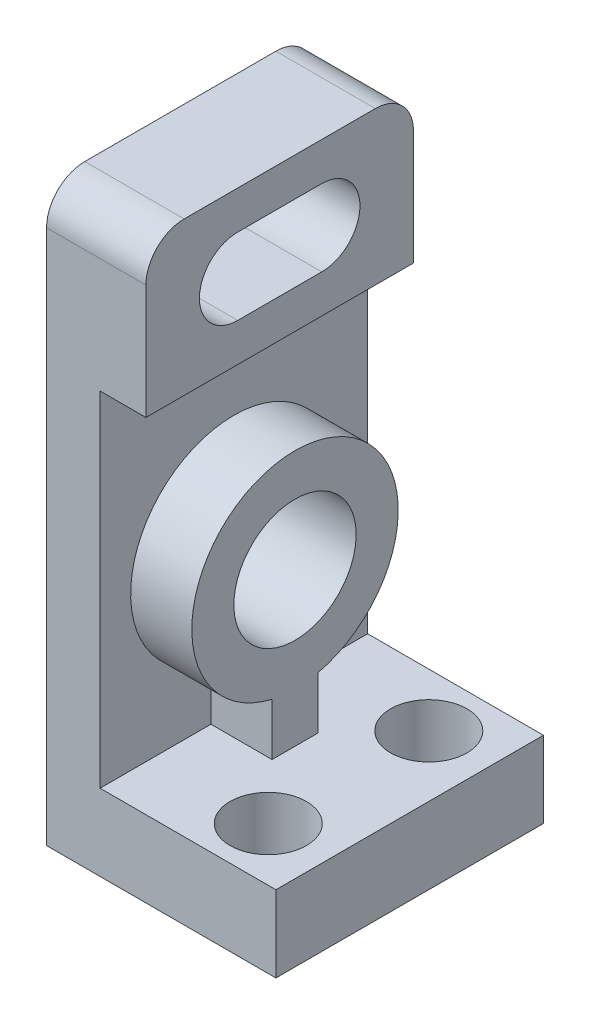
ISO-10303-21;
HEADER;
FILE_DESCRIPTION(('STEP AP214'),'2;1');
FILE_NAME('part.step','',(''),(''),'','','');
FILE_SCHEMA(('AUTOMOTIVE_DESIGN { 1 0 10303 214 1 1 1 1 }'));
ENDSEC;
DATA;
#1=APPLICATION_CONTEXT('core data for automotive mechanical design processes');
#2=APPLICATION_PROTOCOL_DEFINITION('international standard','automotive_design',2000,#1);
#3=PRODUCT_CONTEXT('',#1,'mechanical');
#4=PRODUCT('Part','Part','',(#3));
#5=PRODUCT_RELATED_PRODUCT_CATEGORY('part','',(#4));
#6=PRODUCT_DEFINITION_FORMATION('','',#4);
#7=PRODUCT_DEFINITION_CONTEXT('part definition',#1,'design');
#8=PRODUCT_DEFINITION('design','',#6,#7);
#9=PRODUCT_DEFINITION_SHAPE('','',#8);
#10=(LENGTH_UNIT() NAMED_UNIT(*) SI_UNIT(.MILLI.,.METRE.));
#11=(NAMED_UNIT(*) PLANE_ANGLE_UNIT() SI_UNIT($,.RADIAN.));
#12=(NAMED_UNIT(*) SI_UNIT($,.STERADIAN.) SOLID_ANGLE_UNIT());
#13=UNCERTAINTY_MEASURE_WITH_UNIT(LENGTH_MEASURE(1.E-05),#10,'distance_accuracy_value','');
#14=(GEOMETRIC_REPRESENTATION_CONTEXT(3) GLOBAL_UNCERTAINTY_ASSIGNED_CONTEXT((#13)) GLOBAL_UNIT_ASSIGNED_CONTEXT((#10,
#11,#12)) REPRESENTATION_CONTEXT('',''));
#15=CARTESIAN_POINT('',(0.,0.,0.));
#16=DIRECTION('',(0.,0.,1.));
#17=DIRECTION('',(1.,0.,0.));
#18=AXIS2_PLACEMENT_3D('',#15,#16,#17);
#19=CARTESIAN_POINT('',(7.,10.,17.5));
#20=DIRECTION('',(0.,-1.,0.));
#21=DIRECTION('',(0.,0.,-1.));
#22=AXIS2_PLACEMENT_3D('',#19,#20,#21);
#23=PLANE('',#22);
#24=CARTESIAN_POINT('',(22.,10.,-10.5));
#25=DIRECTION('',(0.,1.,0.));
#26=DIRECTION('',(0.,0.,1.));
#27=AXIS2_PLACEMENT_3D('',#24,#25,#26);
#28=CIRCLE('',#27,5.);
#29=CARTESIAN_POINT('',(22.,10.,-5.5));
#30=VERTEX_POINT('',#29);
#31=EDGE_CURVE('E244',#30,#30,#28,.T.);
#32=ORIENTED_EDGE('',*,*,#31,.F.);
#33=EDGE_LOOP('',(#32));
#34=FACE_BOUND('',#33,.T.);
#35=CARTESIAN_POINT('',(22.,10.,10.5));
#36=DIRECTION('',(0.,1.,0.));
#37=DIRECTION('',(0.,0.,1.));
#38=AXIS2_PLACEMENT_3D('',#35,#36,#37);
#39=CIRCLE('',#38,5.);
#40=CARTESIAN_POINT('',(22.,10.,15.5));
#41=VERTEX_POINT('',#40);
#42=EDGE_CURVE('E236',#41,#41,#39,.T.);
#43=ORIENTED_EDGE('',*,*,#42,.F.);
#44=EDGE_LOOP('',(#43));
#45=FACE_BOUND('',#44,.T.);
#46=DIRECTION('',(-1.,0.,0.));
#47=VECTOR('',#46,1.);
#48=CARTESIAN_POINT('',(15.,10.,-3.));
#49=LINE('',#48,#47);
#50=CARTESIAN_POINT('',(15.,10.,-3.));
#51=VERTEX_POINT('',#50);
#52=CARTESIAN_POINT('',(7.,10.,-3.));
#53=VERTEX_POINT('',#52);
#54=EDGE_CURVE('E226',#51,#53,#49,.T.);
#55=ORIENTED_EDGE('',*,*,#54,.F.);
#56=DIRECTION('',(0.,0.,-1.));
#57=VECTOR('',#56,1.);
#58=CARTESIAN_POINT('',(15.,10.,3.));
#59=LINE('',#58,#57);
#60=CARTESIAN_POINT('',(15.,10.,3.));
#61=VERTEX_POINT('',#60);
#62=EDGE_CURVE('E212',#61,#51,#59,.T.);
#63=ORIENTED_EDGE('',*,*,#62,.F.);
#64=DIRECTION('',(-1.,0.,0.));
#65=VECTOR('',#64,1.);
#66=CARTESIAN_POINT('',(15.,10.,3.));
#67=LINE('',#66,#65);
#68=CARTESIAN_POINT('',(7.,10.,3.));
#69=VERTEX_POINT('',#68);
#70=EDGE_CURVE('E231',#61,#69,#67,.T.);
#71=ORIENTED_EDGE('',*,*,#70,.T.);
#72=DIRECTION('',(0.,0.,-1.));
#73=VECTOR('',#72,1.);
#74=CARTESIAN_POINT('',(7.,10.,17.5));
#75=LINE('',#74,#73);
#76=CARTESIAN_POINT('',(7.,10.,17.5));
#77=VERTEX_POINT('',#76);
#78=EDGE_CURVE('E300',#77,#69,#75,.T.);
#79=ORIENTED_EDGE('',*,*,#78,.F.);
#80=DIRECTION('',(-1.,0.,0.));
#81=VECTOR('',#80,1.);
#82=CARTESIAN_POINT('',(7.,10.,17.5));
#83=LINE('',#82,#81);
#84=CARTESIAN_POINT('',(30.,10.,17.5));
#85=VERTEX_POINT('',#84);
#86=EDGE_CURVE('E258',#85,#77,#83,.T.);
#87=ORIENTED_EDGE('',*,*,#86,.F.);
#88=DIRECTION('',(0.,0.,-1.));
#89=VECTOR('',#88,1.);
#90=CARTESIAN_POINT('',(30.,10.,17.5));
#91=LINE('',#90,#89);
#92=CARTESIAN_POINT('',(30.,10.,-17.5));
#93=VERTEX_POINT('',#92);
#94=EDGE_CURVE('E304',#85,#93,#91,.T.);
#95=ORIENTED_EDGE('',*,*,#94,.T.);
#96=DIRECTION('',(-1.,0.,0.));
#97=VECTOR('',#96,1.);
#98=CARTESIAN_POINT('',(7.,10.,-17.5));
#99=LINE('',#98,#97);
#100=CARTESIAN_POINT('',(7.,10.,-17.5));
#101=VERTEX_POINT('',#100);
#102=EDGE_CURVE('E275',#93,#101,#99,.T.);
#103=ORIENTED_EDGE('',*,*,#102,.T.);
#104=EDGE_CURVE('E299',#53,#101,#75,.T.);
#105=ORIENTED_EDGE('',*,*,#104,.F.);
#106=EDGE_LOOP('',(#55,#63,#71,#79,#87,#95,#103,#105));
#107=FACE_BOUND('',#106,.T.);
#108=ADVANCED_FACE('F39',(#34,#45,#107),#23,.F.);
#109=CARTESIAN_POINT('',(30.,0.,17.5));
#110=DIRECTION('',(0.,1.,0.));
#111=DIRECTION('',(0.,0.,1.));
#112=AXIS2_PLACEMENT_3D('',#109,#110,#111);
#113=PLANE('',#112);
#114=CARTESIAN_POINT('',(22.,0.,10.5));
#115=DIRECTION('',(0.,1.,0.));
#116=DIRECTION('',(0.,0.,1.));
#117=AXIS2_PLACEMENT_3D('',#114,#115,#116);
#118=CIRCLE('',#117,5.);
#119=CARTESIAN_POINT('',(22.,0.,15.5));
#120=VERTEX_POINT('',#119);
#121=EDGE_CURVE('E242',#120,#120,#118,.F.);
#122=ORIENTED_EDGE('',*,*,#121,.F.);
#123=EDGE_LOOP('',(#122));
#124=FACE_BOUND('',#123,.T.);
#125=CARTESIAN_POINT('',(22.,0.,-10.5));
#126=DIRECTION('',(0.,1.,0.));
#127=DIRECTION('',(0.,0.,1.));
#128=AXIS2_PLACEMENT_3D('',#125,#126,#127);
#129=CIRCLE('',#128,5.);
#130=CARTESIAN_POINT('',(22.,0.,-5.5));
#131=VERTEX_POINT('',#130);
#132=EDGE_CURVE('E240',#131,#131,#129,.F.);
#133=ORIENTED_EDGE('',*,*,#132,.F.);
#134=EDGE_LOOP('',(#133));
#135=FACE_BOUND('',#134,.T.);
#136=DIRECTION('',(1.,0.,0.));
#137=VECTOR('',#136,1.);
#138=CARTESIAN_POINT('',(30.,0.,-17.5));
#139=LINE('',#138,#137);
#140=CARTESIAN_POINT('',(0.,0.,-17.5));
#141=VERTEX_POINT('',#140);
#142=CARTESIAN_POINT('',(30.,0.,-17.5));
#143=VERTEX_POINT('',#142);
#144=EDGE_CURVE('E243',#141,#143,#139,.T.);
#145=ORIENTED_EDGE('',*,*,#144,.T.);
#146=DIRECTION('',(0.,0.,-1.));
#147=VECTOR('',#146,1.);
#148=CARTESIAN_POINT('',(30.,0.,17.5));
#149=LINE('',#148,#147);
#150=CARTESIAN_POINT('',(30.,0.,17.5));
#151=VERTEX_POINT('',#150);
#152=EDGE_CURVE('E303',#151,#143,#149,.T.);
#153=ORIENTED_EDGE('',*,*,#152,.F.);
#154=DIRECTION('',(1.,0.,0.));
#155=VECTOR('',#154,1.);
#156=CARTESIAN_POINT('',(30.,0.,17.5));
#157=LINE('',#156,#155);
#158=CARTESIAN_POINT('',(0.,0.,17.5));
#159=VERTEX_POINT('',#158);
#160=EDGE_CURVE('E247',#159,#151,#157,.T.);
#161=ORIENTED_EDGE('',*,*,#160,.F.);
#162=DIRECTION('',(0.,0.,-1.));
#163=VECTOR('',#162,1.);
#164=CARTESIAN_POINT('',(0.,0.,17.5));
#165=LINE('',#164,#163);
#166=EDGE_CURVE('E270',#159,#141,#165,.T.);
#167=ORIENTED_EDGE('',*,*,#166,.T.);
#168=EDGE_LOOP('',(#145,#153,#161,#167));
#169=FACE_BOUND('',#168,.T.);
#170=ADVANCED_FACE('F341',(#124,#135,#169),#113,.F.);
#171=CARTESIAN_POINT('',(30.,10.,17.5));
#172=DIRECTION('',(-1.,0.,0.));
#173=DIRECTION('',(0.,0.,1.));
#174=AXIS2_PLACEMENT_3D('',#171,#172,#173);
#175=PLANE('',#174);
#176=DIRECTION('',(0.,1.,0.));
#177=VECTOR('',#176,1.);
#178=CARTESIAN_POINT('',(30.,10.,-17.5));
#179=LINE('',#178,#177);
#180=EDGE_CURVE('E269',#143,#93,#179,.T.);
#181=ORIENTED_EDGE('',*,*,#180,.T.);
#182=ORIENTED_EDGE('',*,*,#94,.F.);
#183=DIRECTION('',(0.,1.,0.));
#184=VECTOR('',#183,1.);
#185=CARTESIAN_POINT('',(30.,10.,17.5));
#186=LINE('',#185,#184);
#187=EDGE_CURVE('E251',#151,#85,#186,.T.);
#188=ORIENTED_EDGE('',*,*,#187,.F.);
#189=ORIENTED_EDGE('',*,*,#152,.T.);
#190=EDGE_LOOP('',(#181,#182,#188,#189));
#191=FACE_BOUND('',#190,.T.);
#192=ADVANCED_FACE('F368',(#191),#175,.F.);
#193=CARTESIAN_POINT('',(6.99999999999999,55.,17.5));
#194=DIRECTION('',(-1.,0.,0.));
#195=DIRECTION('',(0.,-1.,0.));
#196=AXIS2_PLACEMENT_3D('',#193,#194,#195);
#197=PLANE('',#196);
#198=DIRECTION('',(0.,1.,0.));
#199=VECTOR('',#198,1.);
#200=CARTESIAN_POINT('',(7.,16.8375534189118,-3.));
#201=LINE('',#200,#199);
#202=CARTESIAN_POINT('',(7.,16.8375534189118,-3.));
#203=VERTEX_POINT('',#202);
#204=EDGE_CURVE('E211',#53,#203,#201,.T.);
#205=ORIENTED_EDGE('',*,*,#204,.F.);
#206=ORIENTED_EDGE('',*,*,#104,.T.);
#207=DIRECTION('',(0.,1.,0.));
#208=VECTOR('',#207,1.);
#209=CARTESIAN_POINT('',(6.99999999999999,55.,-17.5));
#210=LINE('',#209,#208);
#211=CARTESIAN_POINT('',(6.99999999999999,55.,-17.5));
#212=VERTEX_POINT('',#211);
#213=EDGE_CURVE('E274',#101,#212,#210,.T.);
#214=ORIENTED_EDGE('',*,*,#213,.T.);
#215=DIRECTION('',(0.,0.,-1.));
#216=VECTOR('',#215,1.);
#217=CARTESIAN_POINT('',(6.99999999999999,55.,17.5));
#218=LINE('',#217,#216);
#219=CARTESIAN_POINT('',(6.99999999999999,55.,17.5));
#220=VERTEX_POINT('',#219);
#221=EDGE_CURVE('E294',#220,#212,#218,.T.);
#222=ORIENTED_EDGE('',*,*,#221,.F.);
#223=DIRECTION('',(0.,1.,0.));
#224=VECTOR('',#223,1.);
#225=CARTESIAN_POINT('',(6.99999999999999,55.,17.5));
#226=LINE('',#225,#224);
#227=EDGE_CURVE('E256',#77,#220,#226,.T.);
#228=ORIENTED_EDGE('',*,*,#227,.F.);
#229=ORIENTED_EDGE('',*,*,#78,.T.);
#230=DIRECTION('',(0.,-1.,0.));
#231=VECTOR('',#230,1.);
#232=CARTESIAN_POINT('',(7.,16.8375534189118,3.));
#233=LINE('',#232,#231);
#234=CARTESIAN_POINT('',(7.,16.8375534189118,3.));
#235=VERTEX_POINT('',#234);
#236=EDGE_CURVE('E225',#235,#69,#233,.T.);
#237=ORIENTED_EDGE('',*,*,#236,.F.);
#238=CARTESIAN_POINT('',(7.,30.,0.));
#239=DIRECTION('',(1.,0.,0.));
#240=DIRECTION('',(0.,1.,0.));
#241=AXIS2_PLACEMENT_3D('',#238,#239,#240);
#242=CIRCLE('',#241,13.5);
#243=EDGE_CURVE('E206',#203,#235,#242,.T.);
#244=ORIENTED_EDGE('',*,*,#243,.F.);
#245=EDGE_LOOP('',(#205,#206,#214,#222,#228,#229,#237,#244));
#246=FACE_BOUND('',#245,.T.);
#247=ADVANCED_FACE('F358',(#246),#197,.F.);
#248=CARTESIAN_POINT('',(13.,55.,17.5));
#249=DIRECTION('',(0.,1.,0.));
#250=DIRECTION('',(0.,0.,1.));
#251=AXIS2_PLACEMENT_3D('',#248,#249,#250);
#252=PLANE('',#251);
#253=DIRECTION('',(1.,0.,0.));
#254=VECTOR('',#253,1.);
#255=CARTESIAN_POINT('',(13.,55.,-17.5));
#256=LINE('',#255,#254);
#257=CARTESIAN_POINT('',(13.,55.,-17.5));
#258=VERTEX_POINT('',#257);
#259=EDGE_CURVE('E280',#212,#258,#256,.T.);
#260=ORIENTED_EDGE('',*,*,#259,.T.);
#261=DIRECTION('',(0.,0.,-1.));
#262=VECTOR('',#261,1.);
#263=CARTESIAN_POINT('',(13.,55.,17.5));
#264=LINE('',#263,#262);
#265=CARTESIAN_POINT('',(13.,55.,17.5));
#266=VERTEX_POINT('',#265);
#267=EDGE_CURVE('E292',#266,#258,#264,.T.);
#268=ORIENTED_EDGE('',*,*,#267,.F.);
#269=DIRECTION('',(1.,0.,0.));
#270=VECTOR('',#269,1.);
#271=CARTESIAN_POINT('',(13.,55.,17.5));
#272=LINE('',#271,#270);
#273=EDGE_CURVE('E257',#220,#266,#272,.T.);
#274=ORIENTED_EDGE('',*,*,#273,.F.);
#275=ORIENTED_EDGE('',*,*,#221,.T.);
#276=EDGE_LOOP('',(#260,#268,#274,#275));
#277=FACE_BOUND('',#276,.T.);
#278=ADVANCED_FACE('F353',(#277),#252,.F.);
#279=CARTESIAN_POINT('',(13.,75.,17.5));
#280=DIRECTION('',(-1.,0.,0.));
#281=DIRECTION('',(0.,-1.,0.));
#282=AXIS2_PLACEMENT_3D('',#279,#280,#281);
#283=PLANE('',#282);
#284=DIRECTION('',(0.,0.,-1.));
#285=VECTOR('',#284,1.);
#286=CARTESIAN_POINT('',(13.,60.,5.5));
#287=LINE('',#286,#285);
#288=CARTESIAN_POINT('',(13.,60.,5.5));
#289=VERTEX_POINT('',#288);
#290=CARTESIAN_POINT('',(13.,60.,-5.5));
#291=VERTEX_POINT('',#290);
#292=EDGE_CURVE('E187',#289,#291,#287,.T.);
#293=ORIENTED_EDGE('',*,*,#292,.F.);
#294=CARTESIAN_POINT('',(13.,65.,5.5));
#295=DIRECTION('',(1.,0.,0.));
#296=DIRECTION('',(0.,1.,0.));
#297=AXIS2_PLACEMENT_3D('',#294,#295,#296);
#298=CIRCLE('',#297,5.);
#299=CARTESIAN_POINT('',(13.,70.,5.5));
#300=VERTEX_POINT('',#299);
#301=EDGE_CURVE('E53',#300,#289,#298,.T.);
#302=ORIENTED_EDGE('',*,*,#301,.F.);
#303=DIRECTION('',(0.,0.,1.));
#304=VECTOR('',#303,1.);
#305=CARTESIAN_POINT('',(13.,70.,5.5));
#306=LINE('',#305,#304);
#307=CARTESIAN_POINT('',(13.,70.,-5.5));
#308=VERTEX_POINT('',#307);
#309=EDGE_CURVE('E174',#308,#300,#306,.T.);
#310=ORIENTED_EDGE('',*,*,#309,.F.);
#311=CARTESIAN_POINT('',(13.,65.,-5.5));
#312=DIRECTION('',(1.,0.,0.));
#313=DIRECTION('',(0.,1.,0.));
#314=AXIS2_PLACEMENT_3D('',#311,#312,#313);
#315=CIRCLE('',#314,5.);
#316=EDGE_CURVE('E191',#291,#308,#315,.T.);
#317=ORIENTED_EDGE('',*,*,#316,.F.);
#318=EDGE_LOOP('',(#293,#302,#310,#317));
#319=FACE_BOUND('',#318,.T.);
#320=DIRECTION('',(0.,1.,0.));
#321=VECTOR('',#320,1.);
#322=CARTESIAN_POINT('',(13.,75.,-17.5));
#323=LINE('',#322,#321);
#324=CARTESIAN_POINT('',(13.,70.,-17.5));
#325=VERTEX_POINT('',#324);
#326=EDGE_CURVE('E276',#258,#325,#323,.T.);
#327=ORIENTED_EDGE('',*,*,#326,.T.);
#328=CARTESIAN_POINT('',(13.,70.,-12.5));
#329=DIRECTION('',(-1.,0.,0.));
#330=DIRECTION('',(0.,-1.,0.));
#331=AXIS2_PLACEMENT_3D('',#328,#329,#330);
#332=CIRCLE('',#331,5.);
#333=CARTESIAN_POINT('',(13.,75.,-12.5));
#334=VERTEX_POINT('',#333);
#335=EDGE_CURVE('E50',#325,#334,#332,.F.);
#336=ORIENTED_EDGE('',*,*,#335,.T.);
#337=DIRECTION('',(0.,0.,-1.));
#338=VECTOR('',#337,1.);
#339=CARTESIAN_POINT('',(13.,75.,17.5));
#340=LINE('',#339,#338);
#341=CARTESIAN_POINT('',(13.,75.,12.5));
#342=VERTEX_POINT('',#341);
#343=EDGE_CURVE('E290',#342,#334,#340,.T.);
#344=ORIENTED_EDGE('',*,*,#343,.F.);
#345=CARTESIAN_POINT('',(13.,70.,12.5));
#346=DIRECTION('',(-1.,0.,0.));
#347=DIRECTION('',(0.,-1.,0.));
#348=AXIS2_PLACEMENT_3D('',#345,#346,#347);
#349=CIRCLE('',#348,5.);
#350=CARTESIAN_POINT('',(13.,70.,17.5));
#351=VERTEX_POINT('',#350);
#352=EDGE_CURVE('E318',#342,#351,#349,.F.);
#353=ORIENTED_EDGE('',*,*,#352,.T.);
#354=DIRECTION('',(0.,1.,0.));
#355=VECTOR('',#354,1.);
#356=CARTESIAN_POINT('',(13.,75.,17.5));
#357=LINE('',#356,#355);
#358=EDGE_CURVE('E265',#266,#351,#357,.T.);
#359=ORIENTED_EDGE('',*,*,#358,.F.);
#360=ORIENTED_EDGE('',*,*,#267,.T.);
#361=EDGE_LOOP('',(#327,#336,#344,#353,#359,#360));
#362=FACE_BOUND('',#361,.T.);
#363=ADVANCED_FACE('F325',(#319,#362),#283,.F.);
#364=CARTESIAN_POINT('',(0.,75.,17.5));
#365=DIRECTION('',(0.,-1.,0.));
#366=DIRECTION('',(0.,0.,-1.));
#367=AXIS2_PLACEMENT_3D('',#364,#365,#366);
#368=PLANE('',#367);
#369=ORIENTED_EDGE('',*,*,#343,.T.);
#370=DIRECTION('',(-1.,0.,0.));
#371=VECTOR('',#370,1.);
#372=CARTESIAN_POINT('',(0.,75.,-12.5));
#373=LINE('',#372,#371);
#374=CARTESIAN_POINT('',(0.,75.,-12.5));
#375=VERTEX_POINT('',#374);
#376=EDGE_CURVE('E310',#334,#375,#373,.T.);
#377=ORIENTED_EDGE('',*,*,#376,.T.);
#378=DIRECTION('',(0.,0.,-1.));
#379=VECTOR('',#378,1.);
#380=CARTESIAN_POINT('',(0.,75.,17.5));
#381=LINE('',#380,#379);
#382=CARTESIAN_POINT('',(0.,75.,12.5));
#383=VERTEX_POINT('',#382);
#384=EDGE_CURVE('E283',#383,#375,#381,.T.);
#385=ORIENTED_EDGE('',*,*,#384,.F.);
#386=DIRECTION('',(-1.,0.,0.));
#387=VECTOR('',#386,1.);
#388=CARTESIAN_POINT('',(0.,75.,12.5));
#389=LINE('',#388,#387);
#390=EDGE_CURVE('E307',#383,#342,#389,.F.);
#391=ORIENTED_EDGE('',*,*,#390,.T.);
#392=EDGE_LOOP('',(#369,#377,#385,#391));
#393=FACE_BOUND('',#392,.T.);
#394=ADVANCED_FACE('F328',(#393),#368,.F.);
#395=CARTESIAN_POINT('',(0.,0.,17.5));
#396=DIRECTION('',(1.,0.,0.));
#397=DIRECTION('',(0.,1.,0.));
#398=AXIS2_PLACEMENT_3D('',#395,#396,#397);
#399=PLANE('',#398);
#400=DIRECTION('',(0.,0.,-1.));
#401=VECTOR('',#400,1.);
#402=CARTESIAN_POINT('',(0.,70.,5.5));
#403=LINE('',#402,#401);
#404=CARTESIAN_POINT('',(0.,70.,5.5));
#405=VERTEX_POINT('',#404);
#406=CARTESIAN_POINT('',(0.,70.,-5.5));
#407=VERTEX_POINT('',#406);
#408=EDGE_CURVE('E184',#405,#407,#403,.T.);
#409=ORIENTED_EDGE('',*,*,#408,.F.);
#410=CARTESIAN_POINT('',(0.,65.,5.5));
#411=DIRECTION('',(1.,0.,0.));
#412=DIRECTION('',(0.,1.,0.));
#413=AXIS2_PLACEMENT_3D('',#410,#411,#412);
#414=CIRCLE('',#413,5.);
#415=CARTESIAN_POINT('',(0.,60.,5.5));
#416=VERTEX_POINT('',#415);
#417=EDGE_CURVE('E167',#416,#405,#414,.F.);
#418=ORIENTED_EDGE('',*,*,#417,.F.);
#419=DIRECTION('',(0.,0.,1.));
#420=VECTOR('',#419,1.);
#421=CARTESIAN_POINT('',(0.,60.,5.5));
#422=LINE('',#421,#420);
#423=CARTESIAN_POINT('',(0.,60.,-5.5));
#424=VERTEX_POINT('',#423);
#425=EDGE_CURVE('E173',#424,#416,#422,.T.);
#426=ORIENTED_EDGE('',*,*,#425,.F.);
#427=CARTESIAN_POINT('',(0.,65.,-5.5));
#428=DIRECTION('',(1.,0.,0.));
#429=DIRECTION('',(0.,1.,0.));
#430=AXIS2_PLACEMENT_3D('',#427,#428,#429);
#431=CIRCLE('',#430,5.);
#432=EDGE_CURVE('E64',#407,#424,#431,.F.);
#433=ORIENTED_EDGE('',*,*,#432,.F.);
#434=EDGE_LOOP('',(#409,#418,#426,#433));
#435=FACE_BOUND('',#434,.T.);
#436=CARTESIAN_POINT('',(0.,30.,0.));
#437=DIRECTION('',(1.,0.,0.));
#438=DIRECTION('',(0.,1.,0.));
#439=AXIS2_PLACEMENT_3D('',#436,#437,#438);
#440=CIRCLE('',#439,8.);
#441=CARTESIAN_POINT('',(0.,38.,0.));
#442=VERTEX_POINT('',#441);
#443=EDGE_CURVE('E180',#442,#442,#440,.F.);
#444=ORIENTED_EDGE('',*,*,#443,.F.);
#445=EDGE_LOOP('',(#444));
#446=FACE_BOUND('',#445,.T.);
#447=ORIENTED_EDGE('',*,*,#384,.T.);
#448=CARTESIAN_POINT('',(0.,70.,-12.5));
#449=DIRECTION('',(1.,0.,0.));
#450=DIRECTION('',(0.,1.,0.));
#451=AXIS2_PLACEMENT_3D('',#448,#449,#450);
#452=CIRCLE('',#451,5.);
#453=CARTESIAN_POINT('',(0.,70.,-17.5));
#454=VERTEX_POINT('',#453);
#455=EDGE_CURVE('E314',#375,#454,#452,.F.);
#456=ORIENTED_EDGE('',*,*,#455,.T.);
#457=DIRECTION('',(0.,-1.,0.));
#458=VECTOR('',#457,1.);
#459=CARTESIAN_POINT('',(0.,0.,-17.5));
#460=LINE('',#459,#458);
#461=EDGE_CURVE('E255',#454,#141,#460,.T.);
#462=ORIENTED_EDGE('',*,*,#461,.T.);
#463=ORIENTED_EDGE('',*,*,#166,.F.);
#464=DIRECTION('',(0.,-1.,0.));
#465=VECTOR('',#464,1.);
#466=CARTESIAN_POINT('',(0.,0.,17.5));
#467=LINE('',#466,#465);
#468=CARTESIAN_POINT('',(0.,70.,17.5));
#469=VERTEX_POINT('',#468);
#470=EDGE_CURVE('E264',#469,#159,#467,.T.);
#471=ORIENTED_EDGE('',*,*,#470,.F.);
#472=CARTESIAN_POINT('',(0.,70.,12.5));
#473=DIRECTION('',(1.,0.,0.));
#474=DIRECTION('',(0.,1.,0.));
#475=AXIS2_PLACEMENT_3D('',#472,#473,#474);
#476=CIRCLE('',#475,5.);
#477=EDGE_CURVE('E315',#469,#383,#476,.F.);
#478=ORIENTED_EDGE('',*,*,#477,.T.);
#479=EDGE_LOOP('',(#447,#456,#462,#463,#471,#478));
#480=FACE_BOUND('',#479,.T.);
#481=ADVANCED_FACE('F182',(#435,#446,#480),#399,.F.);
#482=CARTESIAN_POINT('',(0.,0.,17.5));
#483=DIRECTION('',(0.,0.,-1.));
#484=DIRECTION('',(-1.,0.,0.));
#485=AXIS2_PLACEMENT_3D('',#482,#483,#484);
#486=PLANE('',#485);
#487=ORIENTED_EDGE('',*,*,#358,.T.);
#488=DIRECTION('',(-1.,0.,0.));
#489=VECTOR('',#488,1.);
#490=CARTESIAN_POINT('',(0.,70.,17.5));
#491=LINE('',#490,#489);
#492=EDGE_CURVE('E11',#351,#469,#491,.T.);
#493=ORIENTED_EDGE('',*,*,#492,.T.);
#494=ORIENTED_EDGE('',*,*,#470,.T.);
#495=ORIENTED_EDGE('',*,*,#160,.T.);
#496=ORIENTED_EDGE('',*,*,#187,.T.);
#497=ORIENTED_EDGE('',*,*,#86,.T.);
#498=ORIENTED_EDGE('',*,*,#227,.T.);
#499=ORIENTED_EDGE('',*,*,#273,.T.);
#500=EDGE_LOOP('',(#487,#493,#494,#495,#496,#497,#498,#499));
#501=FACE_BOUND('',#500,.T.);
#502=ADVANCED_FACE('F347',(#501),#486,.F.);
#503=CARTESIAN_POINT('',(0.,0.,-17.5));
#504=DIRECTION('',(0.,0.,-1.));
#505=DIRECTION('',(-1.,0.,0.));
#506=AXIS2_PLACEMENT_3D('',#503,#504,#505);
#507=PLANE('',#506);
#508=ORIENTED_EDGE('',*,*,#461,.F.);
#509=DIRECTION('',(-1.,0.,0.));
#510=VECTOR('',#509,1.);
#511=CARTESIAN_POINT('',(13.,70.,-17.5));
#512=LINE('',#511,#510);
#513=EDGE_CURVE('E316',#454,#325,#512,.F.);
#514=ORIENTED_EDGE('',*,*,#513,.T.);
#515=ORIENTED_EDGE('',*,*,#326,.F.);
#516=ORIENTED_EDGE('',*,*,#259,.F.);
#517=ORIENTED_EDGE('',*,*,#213,.F.);
#518=ORIENTED_EDGE('',*,*,#102,.F.);
#519=ORIENTED_EDGE('',*,*,#180,.F.);
#520=ORIENTED_EDGE('',*,*,#144,.F.);
#521=EDGE_LOOP('',(#508,#514,#515,#516,#517,#518,#519,#520));
#522=FACE_BOUND('',#521,.T.);
#523=ADVANCED_FACE('F340',(#522),#507,.T.);
#524=CARTESIAN_POINT('',(0.,70.,-12.5));
#525=DIRECTION('',(1.,0.,0.));
#526=DIRECTION('',(0.,0.,-1.));
#527=AXIS2_PLACEMENT_3D('',#524,#525,#526);
#528=CYLINDRICAL_SURFACE('',#527,5.);
#529=ORIENTED_EDGE('',*,*,#335,.F.);
#530=ORIENTED_EDGE('',*,*,#513,.F.);
#531=ORIENTED_EDGE('',*,*,#455,.F.);
#532=ORIENTED_EDGE('',*,*,#376,.F.);
#533=EDGE_LOOP('',(#529,#530,#531,#532));
#534=FACE_BOUND('',#533,.T.);
#535=ADVANCED_FACE('F335',(#534),#528,.T.);
#536=CARTESIAN_POINT('',(0.,70.,12.5));
#537=DIRECTION('',(-1.,0.,0.));
#538=DIRECTION('',(0.,0.,1.));
#539=AXIS2_PLACEMENT_3D('',#536,#537,#538);
#540=CYLINDRICAL_SURFACE('',#539,5.);
#541=ORIENTED_EDGE('',*,*,#352,.F.);
#542=ORIENTED_EDGE('',*,*,#390,.F.);
#543=ORIENTED_EDGE('',*,*,#477,.F.);
#544=ORIENTED_EDGE('',*,*,#492,.F.);
#545=EDGE_LOOP('',(#541,#542,#543,#544));
#546=FACE_BOUND('',#545,.T.);
#547=ADVANCED_FACE('F41',(#546),#540,.T.);
#548=CARTESIAN_POINT('',(22.,-0.000999999999999265,-10.5));
#549=DIRECTION('',(0.,1.,0.));
#550=DIRECTION('',(0.,0.,1.));
#551=AXIS2_PLACEMENT_3D('',#548,#549,#550);
#552=CYLINDRICAL_SURFACE('',#551,5.);
#553=ORIENTED_EDGE('',*,*,#31,.T.);
#554=EDGE_LOOP('',(#553));
#555=FACE_BOUND('',#554,.T.);
#556=ORIENTED_EDGE('',*,*,#132,.T.);
#557=EDGE_LOOP('',(#556));
#558=FACE_BOUND('',#557,.T.);
#559=ADVANCED_FACE('F421',(#555,#558),#552,.F.);
#560=CARTESIAN_POINT('',(22.,-0.000999999999999265,10.5));
#561=DIRECTION('',(0.,1.,0.));
#562=DIRECTION('',(0.,0.,1.));
#563=AXIS2_PLACEMENT_3D('',#560,#561,#562);
#564=CYLINDRICAL_SURFACE('',#563,5.);
#565=ORIENTED_EDGE('',*,*,#42,.T.);
#566=EDGE_LOOP('',(#565));
#567=FACE_BOUND('',#566,.T.);
#568=ORIENTED_EDGE('',*,*,#121,.T.);
#569=EDGE_LOOP('',(#568));
#570=FACE_BOUND('',#569,.T.);
#571=ADVANCED_FACE('F385',(#567,#570),#564,.F.);
#572=CARTESIAN_POINT('',(15.,30.,0.));
#573=DIRECTION('',(1.,0.,0.));
#574=DIRECTION('',(0.,1.,0.));
#575=AXIS2_PLACEMENT_3D('',#572,#573,#574);
#576=PLANE('',#575);
#577=CARTESIAN_POINT('',(15.,30.,0.));
#578=DIRECTION('',(1.,0.,0.));
#579=DIRECTION('',(0.,1.,0.));
#580=AXIS2_PLACEMENT_3D('',#577,#578,#579);
#581=CIRCLE('',#580,13.5);
#582=CARTESIAN_POINT('',(15.,16.8375534189118,-3.));
#583=VERTEX_POINT('',#582);
#584=CARTESIAN_POINT('',(15.,16.8375534189118,3.));
#585=VERTEX_POINT('',#584);
#586=EDGE_CURVE('E210',#583,#585,#581,.T.);
#587=ORIENTED_EDGE('',*,*,#586,.T.);
#588=DIRECTION('',(0.,-1.,0.));
#589=VECTOR('',#588,1.);
#590=CARTESIAN_POINT('',(15.,16.8375534189118,3.));
#591=LINE('',#590,#589);
#592=EDGE_CURVE('E209',#585,#61,#591,.T.);
#593=ORIENTED_EDGE('',*,*,#592,.T.);
#594=ORIENTED_EDGE('',*,*,#62,.T.);
#595=DIRECTION('',(0.,1.,0.));
#596=VECTOR('',#595,1.);
#597=CARTESIAN_POINT('',(15.,16.8375534189118,-3.));
#598=LINE('',#597,#596);
#599=EDGE_CURVE('E220',#51,#583,#598,.T.);
#600=ORIENTED_EDGE('',*,*,#599,.T.);
#601=EDGE_LOOP('',(#587,#593,#594,#600));
#602=FACE_BOUND('',#601,.T.);
#603=CARTESIAN_POINT('',(15.,30.,0.));
#604=DIRECTION('',(1.,0.,0.));
#605=DIRECTION('',(0.,1.,0.));
#606=AXIS2_PLACEMENT_3D('',#603,#604,#605);
#607=CIRCLE('',#606,8.);
#608=CARTESIAN_POINT('',(15.,38.,0.));
#609=VERTEX_POINT('',#608);
#610=EDGE_CURVE('E201',#609,#609,#607,.T.);
#611=ORIENTED_EDGE('',*,*,#610,.F.);
#612=EDGE_LOOP('',(#611));
#613=FACE_BOUND('',#612,.T.);
#614=ADVANCED_FACE('F377',(#602,#613),#576,.T.);
#615=CARTESIAN_POINT('',(15.,30.,0.));
#616=DIRECTION('',(-1.,0.,0.));
#617=DIRECTION('',(0.,-1.,0.));
#618=AXIS2_PLACEMENT_3D('',#615,#616,#617);
#619=CYLINDRICAL_SURFACE('',#618,13.5);
#620=ORIENTED_EDGE('',*,*,#243,.T.);
#621=DIRECTION('',(-1.,0.,0.));
#622=VECTOR('',#621,1.);
#623=CARTESIAN_POINT('',(15.,16.8375534189118,3.));
#624=LINE('',#623,#622);
#625=EDGE_CURVE('E233',#585,#235,#624,.T.);
#626=ORIENTED_EDGE('',*,*,#625,.F.);
#627=ORIENTED_EDGE('',*,*,#586,.F.);
#628=DIRECTION('',(-1.,0.,0.));
#629=VECTOR('',#628,1.);
#630=CARTESIAN_POINT('',(15.,16.8375534189118,-3.));
#631=LINE('',#630,#629);
#632=EDGE_CURVE('E218',#583,#203,#631,.T.);
#633=ORIENTED_EDGE('',*,*,#632,.T.);
#634=EDGE_LOOP('',(#620,#626,#627,#633));
#635=FACE_BOUND('',#634,.T.);
#636=ADVANCED_FACE('F373',(#635),#619,.T.);
#637=CARTESIAN_POINT('',(15.,16.8375534189118,3.));
#638=DIRECTION('',(0.,0.,-1.));
#639=DIRECTION('',(0.,1.,0.));
#640=AXIS2_PLACEMENT_3D('',#637,#638,#639);
#641=PLANE('',#640);
#642=ORIENTED_EDGE('',*,*,#236,.T.);
#643=ORIENTED_EDGE('',*,*,#70,.F.);
#644=ORIENTED_EDGE('',*,*,#592,.F.);
#645=ORIENTED_EDGE('',*,*,#625,.T.);
#646=EDGE_LOOP('',(#642,#643,#644,#645));
#647=FACE_BOUND('',#646,.T.);
#648=ADVANCED_FACE('F369',(#647),#641,.F.);
#649=CARTESIAN_POINT('',(15.,16.8375534189118,-3.));
#650=DIRECTION('',(0.,0.,1.));
#651=DIRECTION('',(0.,-1.,0.));
#652=AXIS2_PLACEMENT_3D('',#649,#650,#651);
#653=PLANE('',#652);
#654=ORIENTED_EDGE('',*,*,#204,.T.);
#655=ORIENTED_EDGE('',*,*,#632,.F.);
#656=ORIENTED_EDGE('',*,*,#599,.F.);
#657=ORIENTED_EDGE('',*,*,#54,.T.);
#658=EDGE_LOOP('',(#654,#655,#656,#657));
#659=FACE_BOUND('',#658,.T.);
#660=ADVANCED_FACE('F376',(#659),#653,.F.);
#661=CARTESIAN_POINT('',(15.,30.,0.));
#662=DIRECTION('',(-1.,0.,0.));
#663=DIRECTION('',(0.,-1.,0.));
#664=AXIS2_PLACEMENT_3D('',#661,#662,#663);
#665=CYLINDRICAL_SURFACE('',#664,8.);
#666=ORIENTED_EDGE('',*,*,#610,.T.);
#667=EDGE_LOOP('',(#666));
#668=FACE_BOUND('',#667,.T.);
#669=ORIENTED_EDGE('',*,*,#443,.T.);
#670=EDGE_LOOP('',(#669));
#671=FACE_BOUND('',#670,.T.);
#672=ADVANCED_FACE('F387',(#668,#671),#665,.F.);
#673=CARTESIAN_POINT('',(-0.00100000000003569,65.,5.5));
#674=DIRECTION('',(1.,0.,0.));
#675=DIRECTION('',(0.,1.,0.));
#676=AXIS2_PLACEMENT_3D('',#673,#674,#675);
#677=CYLINDRICAL_SURFACE('',#676,5.);
#678=ORIENTED_EDGE('',*,*,#417,.T.);
#679=DIRECTION('',(1.,0.,0.));
#680=VECTOR('',#679,1.);
#681=CARTESIAN_POINT('',(-0.00100000000003743,70.,5.5));
#682=LINE('',#681,#680);
#683=EDGE_CURVE('E178',#405,#300,#682,.T.);
#684=ORIENTED_EDGE('',*,*,#683,.T.);
#685=ORIENTED_EDGE('',*,*,#301,.T.);
#686=DIRECTION('',(1.,0.,0.));
#687=VECTOR('',#686,1.);
#688=CARTESIAN_POINT('',(-0.00100000000003396,60.,5.5));
#689=LINE('',#688,#687);
#690=EDGE_CURVE('E165',#416,#289,#689,.T.);
#691=ORIENTED_EDGE('',*,*,#690,.F.);
#692=EDGE_LOOP('',(#678,#684,#685,#691));
#693=FACE_BOUND('',#692,.T.);
#694=ADVANCED_FACE('F163',(#693),#677,.F.);
#695=CARTESIAN_POINT('',(-0.00100000000003743,70.,5.5));
#696=DIRECTION('',(0.,1.,0.));
#697=DIRECTION('',(-1.,0.,0.));
#698=AXIS2_PLACEMENT_3D('',#695,#696,#697);
#699=PLANE('',#698);
#700=ORIENTED_EDGE('',*,*,#408,.T.);
#701=DIRECTION('',(1.,0.,0.));
#702=VECTOR('',#701,1.);
#703=CARTESIAN_POINT('',(-0.00100000000003743,70.,-5.5));
#704=LINE('',#703,#702);
#705=EDGE_CURVE('E196',#407,#308,#704,.T.);
#706=ORIENTED_EDGE('',*,*,#705,.T.);
#707=ORIENTED_EDGE('',*,*,#309,.T.);
#708=ORIENTED_EDGE('',*,*,#683,.F.);
#709=EDGE_LOOP('',(#700,#706,#707,#708));
#710=FACE_BOUND('',#709,.T.);
#711=ADVANCED_FACE('F438',(#710),#699,.F.);
#712=CARTESIAN_POINT('',(-0.00100000000003569,65.,-5.5));
#713=DIRECTION('',(1.,0.,0.));
#714=DIRECTION('',(0.,1.,0.));
#715=AXIS2_PLACEMENT_3D('',#712,#713,#714);
#716=CYLINDRICAL_SURFACE('',#715,5.);
#717=ORIENTED_EDGE('',*,*,#432,.T.);
#718=DIRECTION('',(1.,0.,0.));
#719=VECTOR('',#718,1.);
#720=CARTESIAN_POINT('',(-0.00100000000003396,60.,-5.5));
#721=LINE('',#720,#719);
#722=EDGE_CURVE('E172',#424,#291,#721,.T.);
#723=ORIENTED_EDGE('',*,*,#722,.T.);
#724=ORIENTED_EDGE('',*,*,#316,.T.);
#725=ORIENTED_EDGE('',*,*,#705,.F.);
#726=EDGE_LOOP('',(#717,#723,#724,#725));
#727=FACE_BOUND('',#726,.T.);
#728=ADVANCED_FACE('F445',(#727),#716,.F.);
#729=CARTESIAN_POINT('',(-0.00100000000003396,60.,5.5));
#730=DIRECTION('',(0.,-1.,0.));
#731=DIRECTION('',(1.,0.,0.));
#732=AXIS2_PLACEMENT_3D('',#729,#730,#731);
#733=PLANE('',#732);
#734=ORIENTED_EDGE('',*,*,#425,.T.);
#735=ORIENTED_EDGE('',*,*,#690,.T.);
#736=ORIENTED_EDGE('',*,*,#292,.T.);
#737=ORIENTED_EDGE('',*,*,#722,.F.);
#738=EDGE_LOOP('',(#734,#735,#736,#737));
#739=FACE_BOUND('',#738,.T.);
#740=ADVANCED_FACE('F179',(#739),#733,.F.);
#741=CLOSED_SHELL('',(#108,#170,#192,#247,#278,#363,#394,#481,#502,#523,#535,#547,#559,#571,
#614,#636,#648,#660,#672,#694,#711,#728,#740));
#742=MANIFOLD_SOLID_BREP('B2',#741);
#743=ADVANCED_BREP_SHAPE_REPRESENTATION('',(#18,#742),#14);
#744=SHAPE_DEFINITION_REPRESENTATION(#9,#743);
ENDSEC;
END-ISO-10303-21;
